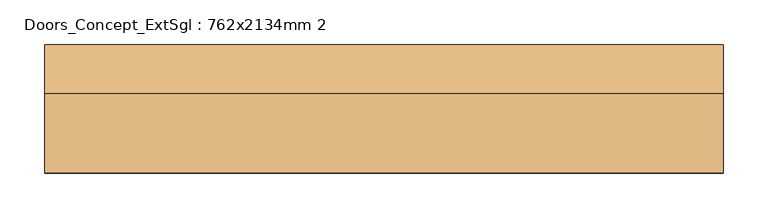
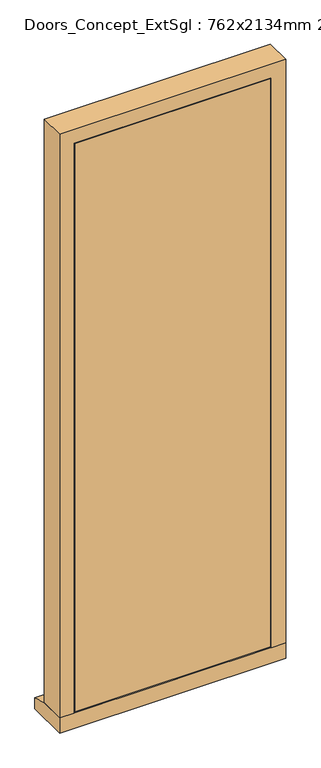
"""IFC4 building model written with IfcOpenShell, lengths in millimetres: door geometry, Doors_Concept_ExtSgl : 762x2134mm 2."""

from ifc_helpers import new_model, si_unit, frame, origin, place, context, project, spatial, polyline, outline, extrude, faceted_brep, source, transform, mapped, element, save


def doors_concept_extsgl_762x2134mm_2_ed5749d6(model_context):
    return source(origin(), model_context, "Body", "SolidModel", [
        faceted_brep([(310.5, 89.3, 54.5), (381.0, 89.3, 54.5), (381.0, 0.3, 54.5), (332.5, 0.3, 54.5), (332.5, 47.3, 54.5), (310.5, 47.3, 54.5), (310.5, 89.3, 2063.1), (-310.5, 89.3, 2063.1), (-310.5, 89.3, 54.5), (-381.0, 89.3, 54.5), (-381.0, 89.3, 2133.6), (381.0, 89.3, 2133.6), (381.0, 0.3, 2133.6), (-381.0, 0.3, 2133.6), (-381.0, 0.3, 54.5), (-332.5, 0.3, 54.5), (-332.5, 0.3, 2085.1), (332.5, 0.3, 2085.1), (332.5, 47.3, 2085.1), (-332.5, 47.3, 2085.1), (-332.5, 47.3, 54.5), (-310.5, 47.3, 54.5), (-310.5, 47.3, 2063.1), (310.5, 47.3, 2063.1)], [[[0, 1, 2, 3, 4, 5]], [[1, 0, 6, 7, 8, 9, 10, 11]], [[2, 1, 11, 12]], [[3, 2, 12, 13, 14, 15, 16, 17]], [[4, 3, 17, 18]], [[5, 4, 18, 19, 20, 21, 22, 23]], [[0, 5, 23, 6]], [[7, 22, 21, 8]], [[8, 21, 20, 15, 14, 9]], [[13, 10, 9, 14]], [[19, 16, 15, 20]], [[12, 11, 10, 13]], [[18, 17, 16, 19]], [[6, 23, 22, 7]]]),
        extrude(outline(polyline([(329.5, 0.3), (-330.4250294, 0.3), (-330.4250294, 44.3), (329.5, 44.3), (329.5, 0.3)])), frame((0.0, 0.0, 58.5), z_axis=(0.0, 0.0, 1.0), x_axis=(1.0, 0.0, 0.0)), (0.0, 0.0, 1.0), 2023.6),
        extrude(outline(polyline([(0.3, 0.0), (0.3, 54.5), (89.3, 54.5), (144.3, 38.5947221), (144.3, 0.0), (0.3, 0.0)])), frame((-381.0, 0.0, 0.0), z_axis=(1.0, 0.0, 0.0), x_axis=(0.0, 1.0, 0.0)), (0.0, 0.0, 1.0), 762.0),
    ])


if __name__ == "__main__":
    model = new_model("IFC4")
    model_context = context("Model", 3, world=origin())
    ifc_project = project(units=[si_unit("LENGTHUNIT", "METRE", prefix="MILLI")], contexts=[model_context])
    site = spatial("IfcSite", under=ifc_project)
    building = spatial("IfcBuilding", under=site)
    placement = place(None, origin())
    doors_concept_extsgl_762x2134mm_2_shape = doors_concept_extsgl_762x2134mm_2_ed5749d6(model_context)
    element("IfcDoor", 1, ObjectType="Doors_Concept_ExtSgl : 762x2134mm 2", at=placement, inside=building, context=model_context, shape_type="MappedRepresentation", body=[
        mapped(doors_concept_extsgl_762x2134mm_2_shape, transform((0.0, 0.0, 0.0), x_axis=(1.0, 0.0, 0.0), y_axis=(0.0, 1.0, 0.0), z_axis=(0.0, 0.0, 1.0))),
    ])
    save(model, "model.ifc")

# Revit data of these elements
# Type "Doors_Concept_ExtSgl : 762x2134mm 2"
#   Type Mark = "17"
#   Type Comments = "External Single"
#   Operation = "SingleSwingRight"
#   Construction Type Id = "SGL"
#   Keynote = "L10"
#   Analytic Construction = "Large single-glazed windows"
#   Visual Light Transmittance = 0.9
#   Thickness = 0' - 1.73228"
#   Solar Heat Gain Coefficient = 0.86
#   Rough Width = 2' - 6"
#   Rough Height = 7' - 0"
#   Heat Transfer Coefficient (U) = 0.979472 BTU/(h·ft²·°F)
#   FrameWidth = 0' - 1.65354"
#   FrameOffset - External = 0' - 0.98425"
#   Height = 7' - 0"
#   Width = 2' - 6"
#   Define Thermal Properties by = 1
#   Function = 1
#   Material Door = Concept
#   Material Frame = Concept
#   Wall Closure = (empty or 0)
#   Assembly Code = ""
# Element 1 (IfcDoor, "Doors_Concept_ExtSgl : 762x2134mm 2")
#   Materials on its faces: "Concept"
# Materials
#   "Concept": colour RGB 128 128 255, transparency 0.5
